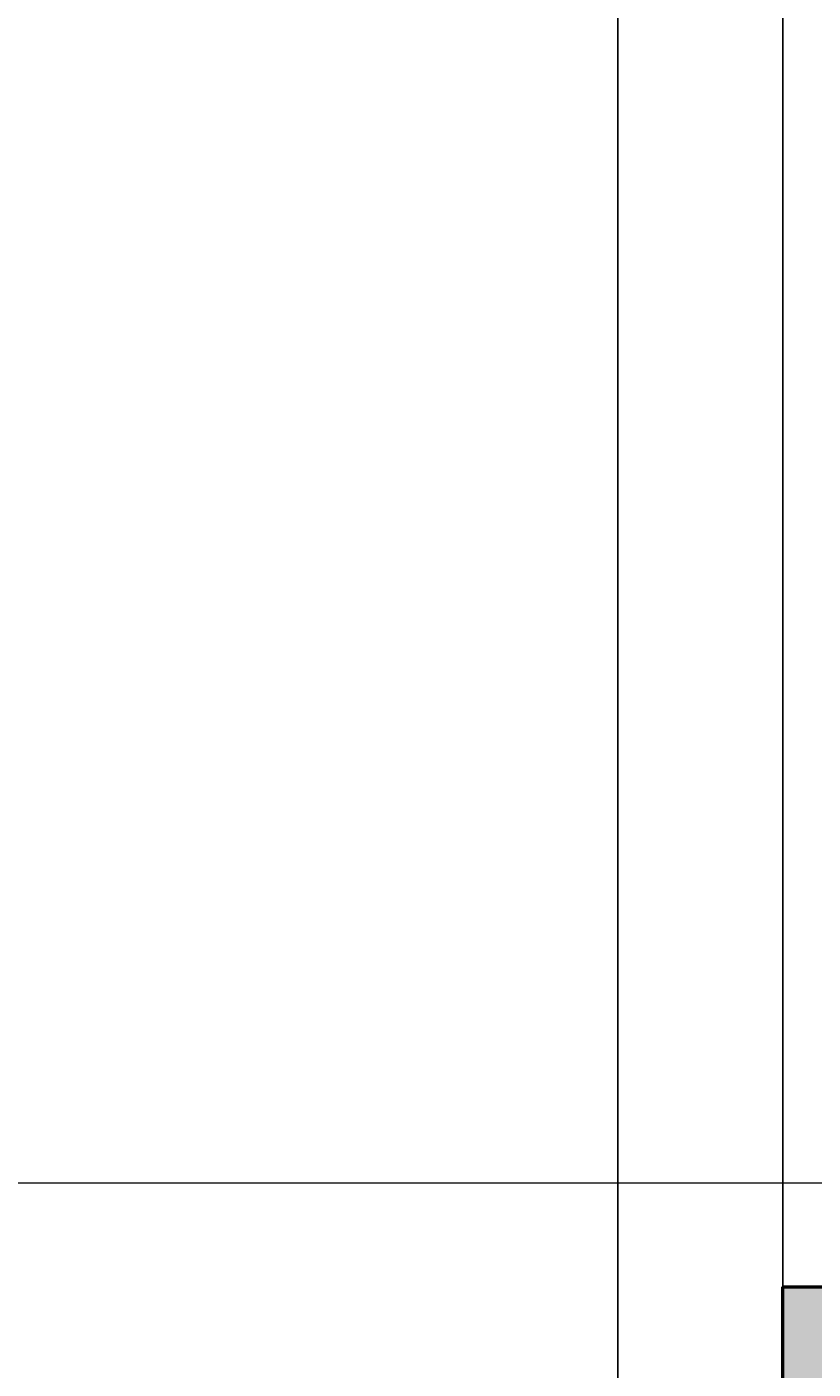
# Model space of a CAD drawing. Units: inches. Extents: x 2231 to 2461, y 2045 to 2455.
# Tile 44 of 95: x 2316 to 2336, y 2185 to 2217. Entities that reach past the tile are written whole.
import ezdxf

# ---------------------------------------------------------------- set-up
doc = ezdxf.new("R2010")
doc.units = ezdxf.units.IN
for name, color, linetype, lineweight in [('A-ANNO-DIMS', 2, 'Continuous', 18), ('A-DOOR', 3, 'Continuous', 25), ('A-FURN', 9, 'Continuous', 18), ('A-WALL', 7, 'Continuous', 50)]:
    doc.layers.add(name, color=color, linetype=linetype, lineweight=lineweight)
doc.layers.add('A-WALL-PATT', color=18, linetype='Continuous', lineweight=13, true_color=0x000000)
doc.styles.get("Standard").update_dxf_attribs({"font": 'arial.ttf'})
doc.dimstyles.get("Standard").update_dxf_attribs({"dimtxt": 0.18, "dimasz": 0.18, "dimexe": 0.18, "dimexo": 0.0625, "dimgap": 0.09, "dimtad": 0, "dimtih": 1, "dimtoh": 1, "dimdec": 4, "dimzin": 0, "dimdsep": 46, "dimtxsty": 'Standard', "dimcen": 0.09, "dimadec": 0, "dimazin": 0, "dimtfac": 1, "dimtdec": 4, "dimtofl": 0, "dimtmove": 0, "dimatfit": 3, "dimfxl": 1, "dimtolj": 1, "dimtzin": 0, "dimarcsym": 0})

# ---------------------------------------------------------------- blocks, each defined once
blk = doc.blocks.new('*U4')
for p, q in [((0, 0), (0, 6)), ((40, 0), (40, 6))]:
    blk.add_line(p, q)
blk.add_lwpolyline([(0, 0), (34.641, -20), (35.516, -18.484), (0.875, 1.516)], close=True)
blk.add_arc((0, 0), 40, 330, 0)
blk = doc.blocks.new('*D50')
at = {"layer": 'A-ANNO-DIMS', "color": 0, "lineweight": -2, "transparency": 16777216}
for p, q in [((2304.794, 2182.895), (2304.794, 2454.645)), ((2334.794, 2182.895), (2334.794, 2454.645)), ((2304.974, 2454.465), (2319.575, 2454.465)), ((2334.614, 2454.465), (2320.012, 2454.465))]:
    blk.add_line(p, q, dxfattribs=at)
at = {"layer": 'A-ANNO-DIMS', "color": 0, "transparency": 16777216}
for points in [[(2304.974, 2454.495), (2304.974, 2454.435), (2304.794, 2454.465)], [(2334.614, 2454.495), (2334.614, 2454.435), (2334.794, 2454.465)]]:
    blk.add_solid(points, dxfattribs=at)
at = {"layer": 'Defpoints', "color": 0, "transparency": 16777216}
for p in [(2334.794, 2454.465), (2304.794, 2182.833), (2334.794, 2182.833)]:
    blk.add_point(p, dxfattribs=at)
at = {"layer": 'A-ANNO-DIMS', "color": 0, "transparency": 16777216, "insert": (2319.794, 2454.465), "char_height": 0.18, "attachment_point": 5}
blk.add_mtext('\\A1;30', dxfattribs=at)
blk = doc.blocks.new('*D51')
at = {"layer": 'A-ANNO-DIMS', "color": 0, "lineweight": -2, "transparency": 16777216}
for p, q in [((2258.794, 2306.77), (2258.794, 2044.803)), ((2330.794, 2306.77), (2330.794, 2044.803)), ((2258.974, 2044.983), (2294.576, 2044.983)), ((2330.614, 2044.983), (2295.011, 2044.983))]:
    blk.add_line(p, q, dxfattribs=at)
at = {"layer": 'A-ANNO-DIMS', "color": 0, "transparency": 16777216}
for points in [[(2258.974, 2045.013), (2258.974, 2044.953), (2258.794, 2044.983)], [(2330.614, 2045.013), (2330.614, 2044.953), (2330.794, 2044.983)]]:
    blk.add_solid(points, dxfattribs=at)
at = {"layer": 'Defpoints', "color": 0, "transparency": 16777216}
for p in [(2258.794, 2306.833), (2330.794, 2306.833), (2330.794, 2044.983)]:
    blk.add_point(p, dxfattribs=at)
at = {"layer": 'A-ANNO-DIMS', "color": 0, "transparency": 16777216, "insert": (2294.794, 2044.983), "char_height": 0.18, "attachment_point": 5}
blk.add_mtext('\\A1;72', dxfattribs=at)
blk = doc.blocks.new('*D52')
at = {"layer": 'A-ANNO-DIMS', "color": 0, "lineweight": -2, "transparency": 16777216}
for p, q in [((2330.794, 2306.77), (2330.794, 2044.803)), ((2360.794, 2306.77), (2360.794, 2044.803)), ((2330.974, 2044.983), (2345.575, 2044.983)), ((2360.614, 2044.983), (2346.012, 2044.983))]:
    blk.add_line(p, q, dxfattribs=at)
at = {"layer": 'A-ANNO-DIMS', "color": 0, "transparency": 16777216}
for points in [[(2330.974, 2045.013), (2330.974, 2044.953), (2330.794, 2044.983)], [(2360.614, 2045.013), (2360.614, 2044.953), (2360.794, 2044.983)]]:
    blk.add_solid(points, dxfattribs=at)
at = {"layer": 'Defpoints', "color": 0, "transparency": 16777216}
for p in [(2330.794, 2306.833), (2360.794, 2306.833), (2360.794, 2044.983)]:
    blk.add_point(p, dxfattribs=at)
at = {"layer": 'A-ANNO-DIMS', "color": 0, "transparency": 16777216, "insert": (2345.794, 2044.983), "char_height": 0.18, "attachment_point": 5}
blk.add_mtext('\\A1;30', dxfattribs=at)
blk = doc.blocks.new('*D65')
at = {"layer": 'A-ANNO-DIMS', "color": 0, "lineweight": -2, "transparency": 16777216}
for p, q in [((2285.635, 2189.285), (2285.635, 2044.803)), ((2340.667, 2189.285), (2340.667, 2044.803)), ((2285.815, 2044.983), (2312.758, 2044.983)), ((2340.487, 2044.983), (2313.545, 2044.983))]:
    blk.add_line(p, q, dxfattribs=at)
at = {"layer": 'A-ANNO-DIMS', "color": 0, "transparency": 16777216}
for points in [[(2285.815, 2045.013), (2285.815, 2044.953), (2285.635, 2044.983)], [(2340.487, 2045.013), (2340.487, 2044.953), (2340.667, 2044.983)]]:
    blk.add_solid(points, dxfattribs=at)
at = {"layer": 'Defpoints', "color": 0, "transparency": 16777216}
for p in [(2285.635, 2189.348), (2340.667, 2189.348), (2340.667, 2044.983)]:
    blk.add_point(p, dxfattribs=at)
at = {"layer": 'A-ANNO-DIMS', "color": 0, "transparency": 16777216, "insert": (2313.151, 2044.983), "char_height": 0.18, "attachment_point": 5}
blk.add_mtext('\\A1;55.03', dxfattribs=at)

msp = doc.modelspace()

# ---------------------------------------------------------------- hatches: boundary and pattern name
at = {"layer": 'A-WALL-PATT'}
h = msp.add_hatch(color=256, dxfattribs=at)
h.dxf.hatch_style = 1
h.paths.add_polyline_path([(2441.7935, 2269.1535), (2432.7935, 2269.1535), (2432.7935, 2186.8328), (2396.7935, 2186.8328), (2396.7935, 2286.8328), (2394.7935, 2286.8328), (2394.7935, 2186.8328), (2334.7935, 2186.8328), (2334.7935, 2182.8328), (2432.7935, 2182.8328), (2432.7935, 2072.8328), (2416.6639, 2072.8328), (2416.6639, 2063.8328), (2441.7935, 2063.8328)])
h.paths.add_polyline_path([(2368.6639, 2072.8328), (2367.04, 2072.8328), (2330.7942, 2072.8328), (2330.7397, 2063.8328), (2368.6639, 2063.8328)])
h.paths.add_polyline_path([(2300.7392, 2068.3328), (2300.7392, 2072.8328), (2298.7935, 2072.8328), (2294.7935, 2072.8328), (2258.7935, 2072.8328), (2258.7935, 2120.8328), (2294.7935, 2120.8328), (2298.7935, 2120.8328), (2298.7935, 2128.8328), (2294.7935, 2128.8328), (2294.7935, 2124.8328), (2258.7935, 2124.8328), (2258.7935, 2182.8328), (2294.7935, 2182.8328), (2294.7935, 2174.8328), (2298.7935, 2174.8328), (2298.7935, 2182.8328), (2304.7935, 2182.8328), (2304.7935, 2186.8328), (2258.7935, 2186.8328), (2258.7935, 2221.999), (2249.7935, 2221.999), (2249.7935, 2063.8328), (2300.7392, 2063.8328)])
h.paths.add_polyline_path([(2391.9338, 2435.8328), (2333.82, 2435.8328), (2333.82, 2426.8328), (2368.7935, 2426.8328), (2368.7935, 2374.9508), (2368.7935, 2370.8328), (2372.3935, 2370.8328), (2372.7935, 2370.8328), (2372.7935, 2426.8328), (2391.9338, 2426.8328)])
h.paths.add_polyline_path([(2441.7935, 2435.8328), (2415.9338, 2435.8328), (2415.9338, 2426.8328), (2432.7935, 2426.8328), (2432.7935, 2334.8328), (2372.7935, 2334.8328), (2372.7935, 2346.8328), (2368.7935, 2346.8328), (2368.7935, 2306.8328), (2360.7935, 2306.8328), (2360.7935, 2302.8328), (2368.7935, 2302.8328), (2372.7935, 2302.8328), (2372.7935, 2330.8328), (2432.7935, 2330.8328), (2432.7935, 2317.1535), (2441.7935, 2317.1535)])
h.paths.add_polyline_path([(2285.82, 2435.8328), (2249.7935, 2435.8328), (2249.7935, 2269.999), (2258.7935, 2269.999), (2258.7935, 2302.8328), (2318.8168, 2302.8328), (2330.7935, 2302.8328), (2330.7935, 2306.8328), (2258.7935, 2306.8328), (2258.7935, 2426.8328), (2285.82, 2426.8328)])

# ---------------------------------------------------------------- linework, layer by layer
at = {"layer": 'A-FURN'}
msp.add_lwpolyline([(2285.6353, 2255.1137), (2285.6353, 2261.3584), (2340.6673, 2261.3584), (2340.6673, 2189.3477), (2285.6353, 2189.3477), (2285.6353, 2195.1137)], dxfattribs=at)
at = {"layer": 'A-WALL'}
for p, q in [((2334.7935, 2182.8328), (2334.7935, 2186.8328)), ((2334.7935, 2186.8328), (2394.7935, 2186.8328))]:
    msp.add_line(p, q, dxfattribs=at)

# ---------------------------------------------------------------- block references
at = {"layer": 'A-DOOR', "xscale": 0.75, "yscale": 0.75, "zscale": 0.75}
msp.add_blockref('*U4', (2304.7935, 2182.8328), dxfattribs=at)

# ---------------------------------------------------------------- dimensions: what is measured, and where the dimension line sits
at = {"layer": 'A-ANNO-DIMS'}
for base, p1, p2, override, picture, middle in [((2334.7935, 2454.4653), (2304.7935, 2182.8328), (2334.7935, 2182.8328), {"dimdec": 0, "dimlfac": 1, "dimrnd": 0, "dimzin": 0, "dimdsep": 46, "dimlunit": 2}, '*D50', (2319.7935, 2454.4653)), ((2330.7935, 2044.9825), (2258.7935, 2306.8328), (2330.7935, 2306.8328), {"dimdec": 0, "dimlfac": 1, "dimrnd": 0, "dimzin": 0, "dimdsep": 46, "dimlunit": 2}, '*D51', (2294.7935, 2044.9825)), ((2360.7935, 2044.9825), (2330.7935, 2306.8328), (2360.7935, 2306.8328), {"dimdec": 0, "dimlfac": 1, "dimrnd": 0, "dimzin": 0, "dimdsep": 46, "dimlunit": 2}, '*D52', (2345.7935, 2044.9825)), ((2340.6673, 2044.9825), (2285.6353, 2189.3477), (2340.6673, 2189.3477), {"dimdec": 2, "dimlfac": 1, "dimrnd": 0, "dimzin": 0, "dimdsep": 46, "dimlunit": 2}, '*D65', (2313.1513, 2044.9825))]:
    dim = msp.add_linear_dim(base=base, p1=p1, p2=p2, dimstyle='Standard', override=override, dxfattribs=at)
    dim.commit()
    dim.dimension.update_dxf_attribs({"geometry": picture, "text_midpoint": middle})

doc.saveas('drawing.dxf')
